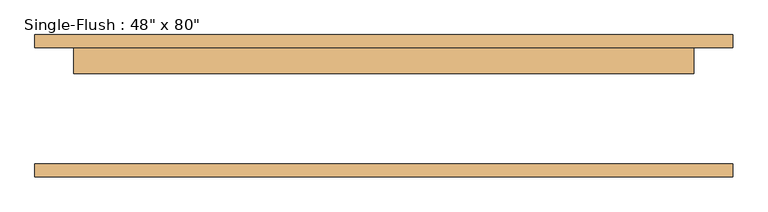
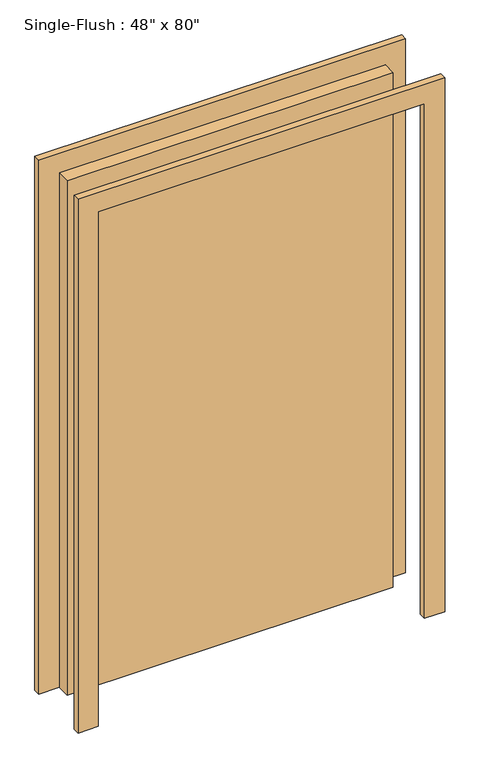
"""IFC4 building model written with IfcOpenShell, lengths in millimetres: door geometry."""

from ifc_helpers import new_model, si_unit, frame, origin, origin_with_axes, place, context, project, spatial, polyline, outline, extrude, source, transform, mapped, element, save


def door_48acaae4(model_context):
    return source(origin(), model_context, "Body", "SweptSolid", [
        extrude(outline(polyline([(2108.2, -685.8), (0.0, -685.8), (0.0, -609.6), (2032.0, -609.6), (2032.0, 609.6), (0.0, 609.6), (0.0, 685.8), (2108.2, 685.8), (2108.2, -685.8)])), frame((0.0, 114.3, 0.0), z_axis=(0.0, 1.0, 0.0), x_axis=(0.0, 0.0, 1.0)), (0.0, 0.0, 1.0), 25.4),
        extrude(outline(polyline([(2108.2, 685.8), (2108.2, -685.8), (0.0, -685.8), (0.0, -609.6), (2032.0, -609.6), (2032.0, 609.6), (0.0, 609.6), (0.0, 685.8), (2108.2, 685.8)])), frame((0.0, -139.7, 0.0), z_axis=(0.0, 1.0, 0.0), x_axis=(0.0, 0.0, 1.0)), (0.0, 0.0, 1.0), 25.4),
        extrude(outline(polyline([(609.6, 63.5), (-609.6, 63.5), (-609.6, 114.3), (609.6, 114.3), (609.6, 63.5)])), origin_with_axes(), (0.0, 0.0, 1.0), 2032.0),
    ])


if __name__ == "__main__":
    model = new_model("IFC4")
    model_context = context("Model", 3, world=origin())
    ifc_project = project(units=[si_unit("LENGTHUNIT", "METRE", prefix="MILLI")], contexts=[model_context])
    site = spatial("IfcSite", under=ifc_project)
    building = spatial("IfcBuilding", under=site)
    placement = place(None, origin())
    door_shape = door_48acaae4(model_context)
    element("IfcDoor", 1, ObjectType="Single-Flush : 48\" x 80\"", at=placement, inside=building, context=model_context, shape_type="MappedRepresentation", body=[
        mapped(door_shape, transform((0.0, 0.0, 0.0), x_axis=(1.0, 0.0, 0.0), y_axis=(0.0, 1.0, 0.0), z_axis=(0.0, 0.0, 1.0))),
    ])
    save(model, "model.ifc")

# Revit data of these elements
# Type "Single-Flush : 48\" x 80\""
#   Type Mark = "5"
#   Construction Type Id = "MDOOR"
#   Assembly Code = "C1020"
#   Analytic Construction = "Metal"
#   Thickness = 0' - 2"
#   Heat Transfer Coefficient (U) = 0.651978 BTU/(h·ft²·°F)
#   Height = 6' - 8"
#   Trim Projection Ext = 0' - 1"
#   Trim Projection Int = 0' - 1"
#   Trim Width = 0' - 3"
#   Width = 4' - 0"
#   Define Thermal Properties by = 1
#   Define Thermal Properties by = 1
#   Door Material = Door - Panel
#   Frame Material = Door - Frame
#   Visual Light Transmittance = 0
#   Solar Heat Gain Coefficient = 0
#   Function = (empty or 0)
#   Wall Closure = (empty or 0)
# Element 1 (IfcDoor, "Single-Flush : 48\" x 80\"")
#   Materials on its faces: "Door - Frame", "Door - Panel"
# Materials
#   "Door - Panel": class "Wood", colour RGB 210 159 95, transparency 0, Cost = 0
#   "Door - Frame": colour RGB 118 70 51, transparency 0, Cost = 0
